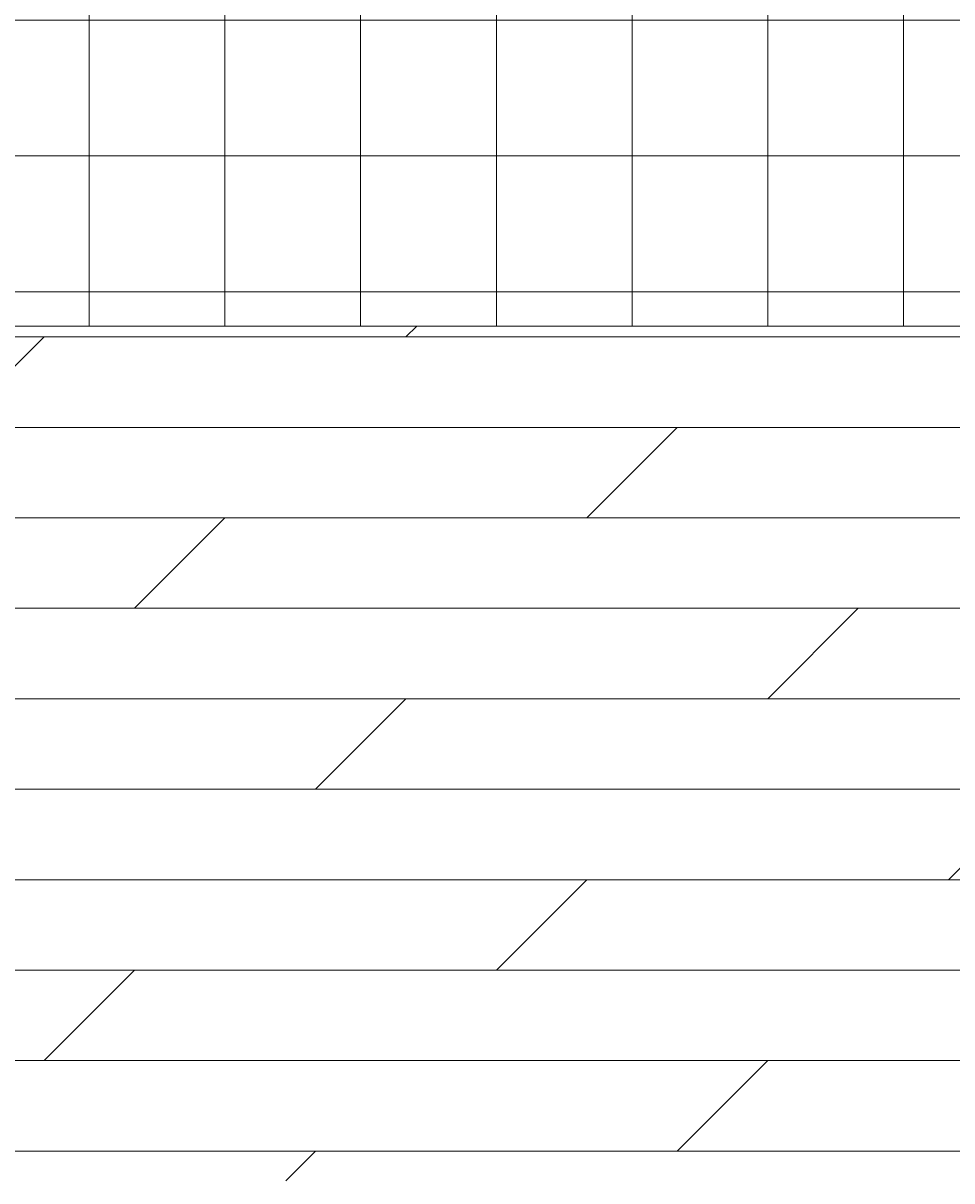
# Model space of a CAD drawing. Units: inches. Extents: x 84 to 1044, y -280 to 906.
# Tile 52 of 105: x 310 to 375, y 709 to 790. Entities that reach past the tile are written whole.
import ezdxf

# ---------------------------------------------------------------- set-up
doc = ezdxf.new("R2010")
doc.units = ezdxf.units.IN
doc.layers.add('A-ANNO-DIMS', color=2, linetype='Continuous', lineweight=18)
doc.layers.add('L-HRDS', color=32, linetype='Continuous', lineweight=18)
doc.layers.add('A-FLOR-PATT', color=251, linetype='Continuous', lineweight=9, true_color=0x705861)
doc.styles.get("Standard").update_dxf_attribs({"font": 'arial.ttf'})
doc.dimstyles.get("Standard").update_dxf_attribs({"dimtxt": 0.18, "dimasz": 0.18, "dimexe": 0.18, "dimexo": 0.0625, "dimgap": 0.09, "dimtad": 0, "dimtih": 1, "dimtoh": 1, "dimdec": 4, "dimzin": 0, "dimdsep": 46, "dimtxsty": 'Standard', "dimcen": 0.09, "dimadec": 0, "dimazin": 0, "dimtfac": 1, "dimtdec": 4, "dimtofl": 0, "dimtmove": 0, "dimatfit": 3, "dimfxl": 1, "dimtolj": 1, "dimtzin": 0, "dimarcsym": 0})

# ---------------------------------------------------------------- blocks, each defined once
blk = doc.blocks.new('*D62')
at = {"layer": 'A-ANNO-DIMS', "color": 0, "lineweight": -2, "transparency": 16777216}
for p, q in [((203.179, 709.183), (203.179, 905.9)), ((203.359, 905.72), (549.232, 905.72)), ((895.894, 905.72), (550.021, 905.72)), ((896.074, 400.183), (896.074, 905.9))]:
    blk.add_line(p, q, dxfattribs=at)
at = {"layer": 'A-ANNO-DIMS', "color": 0, "transparency": 16777216}
for points in [[(203.359, 905.75), (203.359, 905.69), (203.179, 905.72)], [(895.894, 905.75), (895.894, 905.69), (896.074, 905.72)]]:
    blk.add_solid(points, dxfattribs=at)
at = {"layer": 'Defpoints', "color": 0, "transparency": 16777216}
for p in [(896.074, 905.72), (203.179, 709.12), (896.074, 400.12)]:
    blk.add_point(p, dxfattribs=at)
at = {"layer": 'A-ANNO-DIMS', "color": 0, "transparency": 16777216, "insert": (549.627, 905.72), "char_height": 0.18, "attachment_point": 5}
blk.add_mtext('\\A1;692.9', dxfattribs=at)

msp = doc.modelspace()

# ---------------------------------------------------------------- hatches: boundary and pattern name
at = {"layer": 'A-FLOR-PATT', "transparency": 33554597}
h = msp.add_hatch(dxfattribs=at)
h.set_pattern_fill('ANSI37', color=256, scale=3, angle=45)
h.paths.add_polyline_path([(410.074, 847.12), (143.179, 847.12), (143.179, 769.12), (203.179, 769.12), (410.074, 769.12)])
h.paths.add_polyline_path([(254.313, 826.374, -0.414214), (254.257, 823.878, -0.414214), (251.76, 823.934), (244.439, 831.592, 0.3775), (230.555, 830.526, 0.076599), (228.51, 828.052, -0.127919), (230.803, 827.709, -0.121523), (233.469, 828.328, -0.425989), (233.291, 814.163, -0.165541), (230.889, 815.094, -0.016888), (230.578, 814.914), (236.189, 809.046, -0.414214), (236.133, 806.549, -0.414214), (233.636, 806.605, 0.414214), (238.63, 806.493), (246.415, 813.937), (254.201, 821.381, 0.414214)], flags=16)
h.paths.add_polyline_path([(241.241, 801.211), (258.998, 817.357), (267.168, 808.372), (249.545, 792.347)], flags=16)
h.paths.add_polyline_path([(262.121, 832.717, -1), (274.121, 832.717, -1)], flags=16)
h.paths.add_polyline_path([(315.269, 832.717, -1), (327.269, 832.717, -1)], flags=16)
h.paths.add_polyline_path([(322.221, 808.372), (330.392, 817.357), (348.148, 801.211), (339.844, 792.347)], flags=16)
h.paths.add_polyline_path([(344.951, 831.592, -0.372719), (358.711, 830.652), (358.966, 830.408, -0.072384), (360.879, 828.052, -0.103042), (362.667, 827.476, -0.02342), (363.022, 827.039, 0.134832), (360.058, 831.805, 0.419104)], flags=0)
h.paths.add_polyline_path([(355.753, 806.605, -0.414214), (353.257, 806.549, -0.414214), (353.201, 809.046), (358.811, 814.914, 0.234158), (363.536, 814.769, 0.403722), (362.499, 834.358, 0.41788), (342.398, 834.032), (335.076, 826.374, 0.414214), (335.188, 821.381), (342.974, 813.937), (350.76, 806.493, 0.414214)], flags=16)
h = msp.add_hatch(dxfattribs=at)
h.set_pattern_fill('DOLMIT', color=256)
h.paths.add_polyline_path([(896.074, 709.12), (833.074, 709.12), (833.074, 646.12), (833.074, 574.12), (833.074, 511.12), (896.074, 511.12)])
h.paths.add_polyline_path([(386.074, 769.12), (203.179, 769.12), (203.179, 709.12), (287.127, 709.12), (359.127, 709.12), (386.074, 709.12)])

# ---------------------------------------------------------------- linework, layer by layer
at = {"layer": 'L-HRDS'}
msp.add_line((203.179, 769.12), (434.074, 769.12), dxfattribs=at)

# ---------------------------------------------------------------- dimensions: what is measured, and where the dimension line sits
at = {"layer": 'A-ANNO-DIMS'}
dim = msp.add_linear_dim(base=(896.074, 905.72), p1=(203.179, 709.12), p2=(896.074, 400.12), dimstyle='Standard', override={"dimdec": 1, "dimlfac": 1, "dimrnd": 0, "dimzin": 0, "dimdsep": 46, "dimlunit": 2}, dxfattribs=at)
dim.commit()
dim.dimension.update_dxf_attribs({"geometry": '*D62', "text_midpoint": (549.627, 905.72)})

doc.saveas('drawing.dxf')
